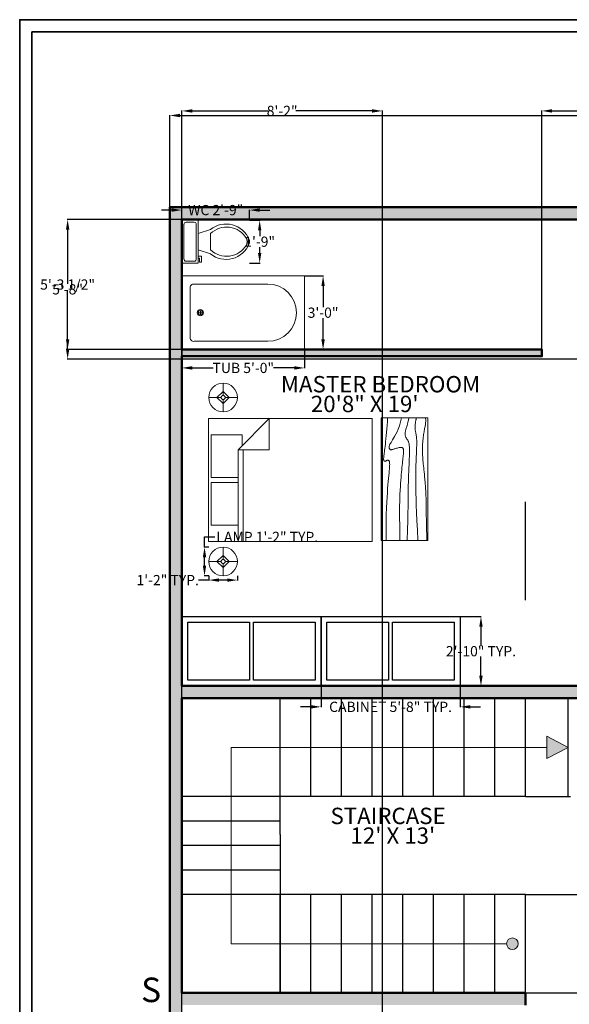
# Model space of a CAD drawing. Units: inches. Extents: x -60 to 743, y -483 to 510.
# Tile 5 of 7: x -60 to 209, y 29 to 510. Entities that reach past the tile are written whole.
import ezdxf

# ---------------------------------------------------------------- set-up
doc = ezdxf.new("R2010")
doc.units = ezdxf.units.IN
doc.header["$MEASUREMENT"] = 0
for name, color, linetype, lineweight in [('A-ANNO-DIMS', 2, 'Continuous', 18), ('A-ANNO-SYMB', 7, 'Continuous', 18), ('A-ANNO-TTLB', 7, 'Continuous', 35), ('A-AREA-IDEN', 7, 'Continuous', 25), ('A-FLOR-CASE', 40, 'Continuous', 25), ('A-FLOR-FIXT', 40, 'Continuous', 18), ('A-WALL-PATT', 30, 'Continuous', 13), ('FURNITURE', 40, 'Continuous', 18), ('STAIRS', 202, 'Continuous', 25), ('WALL BOUNDRY', 10, 'Continuous', 50)]:
    doc.layers.add(name, color=color, linetype=linetype, lineweight=lineweight)
doc.styles.get("Standard").update_dxf_attribs({"font": 'arial.ttf'})
doc.dimstyles.get("Standard").update_dxf_attribs({"dimtxt": 5, "dimasz": 5, "dimexe": 0.18, "dimexo": 0.0625, "dimgap": 0.09, "dimtad": 0, "dimtih": 1, "dimtoh": 1, "dimdec": 1, "dimzin": 0, "dimdsep": 46, "dimlunit": 4, "dimtxsty": 'Standard', "dimcen": 0.09, "dimadec": 0, "dimazin": 0, "dimtfac": 1, "dimtdec": 1, "dimtofl": 0, "dimtmove": 0, "dimatfit": 3, "dimfxl": 1, "dimtolj": 1, "dimtzin": 0, "dimarcsym": 0})

# ---------------------------------------------------------------- blocks, each defined once
blk = doc.blocks.new('Wall Cabinet - 18 x 36 in front')
for p, q in [((17.5, -1.5), (17.5, -16.5)), ((18.5, -16.5), (18.5, -1.5))]:
    blk.add_line(p, q)
blk.add_lwpolyline([(0, -18), (0, 0), (36, 0), (36, -18)], close=True)
for points in [[(17.5, -16.5), (1.5, -16.5), (1.5, -1.5), (17.5, -1.5)], [(18.5, -1.5), (34.5, -1.5), (34.5, -16.5), (18.5, -16.5)]]:
    blk.add_lwpolyline(points)
blk = doc.blocks.new('Bath Tub - 26 x 60 in.')
for p, q in [((8, -18), (10, -18)), ((9, -17), (9, -19))]:
    blk.add_line(p, q)
blk.add_lwpolyline([(0, -36), (0, 0), (60, 0), (60, -36)], close=True)
for points in [[(6, -4), (42, -4)], [(4, -30), (4, -6)], [(42, -32), (6, -32)]]:
    blk.add_lwpolyline(points)
for radius in [1.5, 1]:
    blk.add_circle((9, -18), radius)
for centre, radius, start, end in [((5.75, -5.75), 1.77, 81.8699, 188.1301), ((42, -18), 14, 270, 90), ((5.75, -30.25), 1.77, 171.8699, 278.1301)]:
    blk.add_arc(centre, radius, start, end)
blk = doc.blocks.new('Toilet - top')
for p, q in [((9.5, -6), (9.5, -2)), ((-10, -8.5), (-8, -8.5)), ((-10, -9.5), (-10, -8.5)), ((-7, -9.5), (-10, -9.5)), ((-8, -8.5), (-8, -8)), ((-7, -8), (-7, -9.5)), ((-4, -8), (-6, -14)), ((4, -8), (6, -14)), ((4, -14), (-4, -14))]:
    blk.add_line(p, q)
blk.add_lwpolyline([(10.5, -8), (10.5, 0), (-10.5, 0), (-10.5, -8)], close=True)
for points in [[(-9.5, -2), (-9.5, -6)], [(8.5, -1), (-8.5, -1)], [(-8.5, -7), (8.5, -7)]]:
    blk.add_lwpolyline(points)
for centre, radius, start, end in [((-8.62, -1.88), 0.884, 81.8699, 188.1301), ((8.62, -1.88), 0.884, 351.8699, 98.1301), ((-8.62, -6.12), 0.884, 171.8699, 278.1301), ((8.62, -6.12), 0.884, 261.8699, 8.1301), ((3.52, -21.58), 12.17, 141.4691, 247.9714), ((4.2, -21.82), 11.33, 136.3677, 238.9468), ((-3.52, -21.58), 12.17, 292.0284, 38.5307), ((-4.2, -21.82), 11.33, 301.053, 43.6321), ((0, -27.88), 4, 245.7318, 294.2682), ((0, -29), 4, 254.8605, 285.1395)]:
    blk.add_arc(centre, radius, start, end)
blk = doc.blocks.new('Lamp - Table')
for p, q in [((0, 7), (0, 1)), ((-1, 0), (-7, 0)), ((0, 3), (-3, 0)), ((-3, 0), (0, -3)), ((3, 0), (0, 3)), ((0, -3), (3, 0)), ((1, 0), (7, 0)), ((0, -1), (0, -7))]:
    blk.add_line(p, q)
for radius in [7, 1]:
    blk.add_circle((0, 0), radius)
blk = doc.blocks.new('Bed - Queen')
for p, q in [((0, -80.00003), (0, 0)), ((0, 0), (59.99999, 0)), ((59.99999, 0), (59.99999, -80.00003)), ((7.99999, -1.2), (28.79998, -1.2)), ((7.99999, -14.4), (7.99999, -1.2)), ((28.79998, -1.2), (28.79998, -14.4)), ((31.19999, -1.2), (51.99999, -1.2)), ((31.19999, -14.4), (31.19999, -1.2)), ((51.99999, -1.2), (51.99999, -16.4)), ((0, -14.4), (44.8, -14.4)), ((59.99999, -29.6), (44.8, -14.4)), ((44.8, -14.4), (44.8, -29.6)), ((44.8, -16.8), (0, -16.8)), ((51.99999, -16.4), (46.79936, -16.4)), ((44.8, -29.6), (59.99999, -29.6)), ((59.99999, -80.00003), (0, -80.00003))]:
    blk.add_line(p, q)
blk = doc.blocks.new('*D22')
at = {"layer": 'A-ANNO-DIMS', "color": 0, "lineweight": -2, "transparency": 16777216}
for p, q in [((13.15, 418.48), (13.15, 463.48)), ((18.15, 463.3), (310.31, 463.3)), ((611.15, 463.3), (318.98, 463.3)), ((616.15, 418.48), (616.15, 463.48))]:
    blk.add_line(p, q, dxfattribs=at)
at = {"layer": 'A-ANNO-DIMS', "color": 0, "transparency": 16777216}
for points in [[(18.15, 464.13), (18.15, 462.46), (13.15, 463.3)], [(611.15, 464.13), (611.15, 462.46), (616.15, 463.3)]]:
    blk.add_solid(points, dxfattribs=at)
at = {"layer": 'Defpoints', "color": 0, "transparency": 16777216}
for p in [(616.15, 463.3), (13.15, 418.42), (616.15, 418.42)]:
    blk.add_point(p, dxfattribs=at)
at = {"layer": 'A-ANNO-DIMS', "color": 0, "transparency": 16777216, "insert": (314.65, 463.3), "char_height": 5, "attachment_point": 5}
blk.add_mtext("\\A1;50'", dxfattribs=at)
blk = doc.blocks.new('BENCH-WOOD-60IN')
blk.add_lwpolyline([(22.9143, 0), (22.9143, 60), (0, 60), (0, 0)], close=True)
for points in [[(2.4, 0), (2.418, 4.8155), (2.4688, 9.0302), (2.5477, 12.709), (2.65, 15.9167), (2.7711, 18.7181), (2.9063, 21.1781), (3.0508, 23.3616), (3.2, 25.3333), (3.3495, 27.1477), (3.4958, 28.8172), (3.636, 30.3437), (3.7667, 31.7291), (3.8849, 32.9756), (3.9875, 34.0849), (4.0714, 35.059), (4.1334, 35.9), (4.1711, 36.6114), (4.1854, 37.2041), (4.1779, 37.6906), (4.15, 38.0833), (4.1034, 38.3948), (4.0396, 38.6375), (3.9602, 38.8239), (3.8667, 38.9666), (3.7608, 39.0764), (3.6448, 39.1573), (3.521, 39.2116), (3.3917, 39.2416), (3.2593, 39.2498), (3.1261, 39.2385), (2.9944, 39.21), (2.8667, 39.1666), (2.7447, 39.111), (2.6281, 39.0468), (2.5163, 38.978), (2.4083, 38.9083), (2.3035, 38.8418), (2.201, 38.7823), (2.1001, 38.7337), (2, 38.7), (1.9003, 38.6844), (1.8021, 38.6875), (1.707, 38.7094), (1.6167, 38.75), (1.5326, 38.8094), (1.4563, 38.8875), (1.3893, 38.9844), (1.3333, 39.1), (1.2896, 39.2351), (1.2583, 39.3937), (1.2396, 39.5804), (1.2333, 39.8), (1.2396, 40.057), (1.2583, 40.3562), (1.2896, 40.7023), (1.3333, 41.1), (1.3895, 41.5547), (1.4573, 42.0755), (1.5361, 42.6721), (1.625, 43.3542), (1.7233, 44.1316), (1.8302, 45.014), (1.9449, 46.0114), (2.0667, 47.1333), (2.1947, 48.3862), (2.3281, 49.7625), (2.4663, 51.2513), (2.6083, 52.8416), (2.7535, 54.5226), (2.9011, 56.2833), (3.0501, 58.1127), (3.2, 60)], [(9.2, 0), (9.0858, 6.5759), (9.0365, 11.9385), (9.0418, 16.2527), (9.0917, 19.6833), (9.1759, 22.3952), (9.2844, 24.5531), (9.4069, 26.322), (9.5333, 27.8666), (9.6553, 29.3241), (9.7719, 30.7203), (9.8837, 32.0532), (9.9917, 33.3208), (10.0965, 34.5213), (10.199, 35.6526), (10.2999, 36.7128), (10.4, 37.7), (10.4996, 38.6129), (10.5969, 39.4531), (10.6895, 40.223), (10.775, 40.925), (10.8512, 41.5613), (10.9156, 42.1344), (10.966, 42.6465), (11, 43.1), (11.0158, 43.4976), (11.0136, 43.8437), (10.9942, 44.143), (10.9583, 44.4), (10.9069, 44.6195), (10.8406, 44.8062), (10.7603, 44.9648), (10.6667, 45.1), (10.5598, 45.2155), (10.4365, 45.3114), (10.2929, 45.3871), (10.125, 45.4416), (9.929, 45.4743), (9.7011, 45.4844), (9.4371, 45.4709), (9.1333, 45.4333), (8.7883, 45.3716), (8.4104, 45.2896), (8.0107, 45.1919), (7.6, 45.0833), (7.1893, 44.9685), (6.7896, 44.8521), (6.4117, 44.7388), (6.0667, 44.6333), (5.7628, 44.54), (5.4979, 44.4614), (5.2675, 44.4001), (5.0667, 44.3583), (4.8909, 44.3384), (4.7354, 44.3427), (4.5956, 44.3736), (4.4667, 44.4333), (4.3453, 44.5236), (4.2333, 44.6427), (4.1339, 44.7884), (4.05, 44.9583), (3.9849, 45.1501), (3.9417, 45.3614), (3.9234, 45.59), (3.9333, 45.8333), (3.9749, 46.0915), (4.0531, 46.3734), (4.1736, 46.6906), (4.3417, 47.0542), (4.5629, 47.4756), (4.8427, 47.9661), (5.1866, 48.5372), (5.6, 49.2), (6.0844, 49.9676), (6.625, 50.8594), (7.2031, 51.8965), (7.8, 53.1), (8.3969, 54.491), (8.975, 56.0906), (9.5156, 57.9199), (10, 60)], [(12.8, 0), (12.9322, 5.1847), (13.0323, 9.6213), (13.1059, 13.3963), (13.1583, 16.5958), (13.1952, 19.3063), (13.2219, 21.614), (13.2439, 23.6054), (13.2667, 25.3666), (13.2947, 26.9728), (13.3281, 28.4531), (13.3663, 29.8256), (13.4083, 31.1083), (13.4535, 32.3191), (13.501, 33.476), (13.5501, 34.597), (13.6, 35.7), (13.6497, 36.7984), (13.6979, 37.8875), (13.743, 38.9578), (13.7833, 40), (13.8174, 41.0047), (13.8438, 41.9625), (13.8607, 42.864), (13.8667, 43.7), (13.8604, 44.4631), (13.8417, 45.1552), (13.8104, 45.7801), (13.7667, 46.3416), (13.7104, 46.8439), (13.6417, 47.2906), (13.5604, 47.6858), (13.4667, 48.0333), (13.3608, 48.3375), (13.2448, 48.6042), (13.121, 48.8396), (12.9917, 49.05), (12.8593, 49.2417), (12.7261, 49.4208), (12.5944, 49.5937), (12.4667, 49.7667), (12.3451, 49.9452), (12.2313, 50.1323), (12.1268, 50.3303), (12.0333, 50.5416), (11.9524, 50.7686), (11.8854, 51.0135), (11.8341, 51.2788), (11.8, 51.5666), (11.7843, 51.8785), (11.7865, 52.2116), (11.8059, 52.562), (11.8417, 52.926), (11.8931, 53.2998), (11.9594, 53.6795), (12.0397, 54.0614), (12.1333, 54.4416), (12.2401, 54.8223), (12.3625, 55.2293), (12.5037, 55.6942), (12.6667, 56.2489), (12.8547, 56.9251), (13.0708, 57.7545), (13.3182, 58.7689), (13.6, 60)], [(18, 0), (17.7273, 5.124), (17.5057, 9.6609), (17.3303, 13.6705), (17.1958, 17.2125), (17.0973, 20.3467), (17.0297, 23.1328), (16.9878, 25.6307), (16.9667, 27.9), (16.9617, 29.9928), (16.9703, 31.9302), (16.9907, 33.7254), (17.0208, 35.3917), (17.0588, 36.9423), (17.1026, 38.3906), (17.1503, 39.7499), (17.2, 41.0333), (17.2496, 42.2519), (17.2969, 43.4073), (17.3395, 44.4986), (17.375, 45.525), (17.4012, 46.4858), (17.4156, 47.3802), (17.416, 48.2074), (17.4, 48.9667), (17.3662, 49.6583), (17.3167, 50.2872), (17.2547, 50.8595), (17.1833, 51.3812), (17.1057, 51.8584), (17.025, 52.2971), (16.9443, 52.7034), (16.8667, 53.0833), (16.7951, 53.443), (16.7313, 53.789), (16.6768, 54.128), (16.6334, 54.4666), (16.6024, 54.8115), (16.5854, 55.1693), (16.5841, 55.5465), (16.6, 55.95), (16.6337, 56.3828), (16.6823, 56.8346), (16.7418, 57.2915), (16.8084, 57.7396), (16.878, 58.165), (16.9469, 58.5539), (17.0111, 58.8924), (17.0667, 59.1666), (17.1107, 59.3679), (17.1438, 59.5078), (17.1675, 59.6032), (17.1833, 59.6708), (17.193, 59.7275), (17.1979, 59.7901), (17.1998, 59.8753), (17.2, 60)], [(22.4, 0), (22.2501, 8.0098), (22.1011, 14.4094), (21.9535, 19.4168), (21.8083, 23.25), (21.6663, 26.1269), (21.5281, 28.2656), (21.3947, 29.884), (21.2667, 31.2), (21.1448, 32.3967), (21.0292, 33.5172), (20.9198, 34.5697), (20.8167, 35.5625), (20.7198, 36.5037), (20.6292, 37.4015), (20.5448, 38.2642), (20.4667, 39.1), (20.3951, 39.9164), (20.3313, 40.7187), (20.2768, 41.5117), (20.2333, 42.3), (20.2024, 43.0883), (20.1854, 43.8812), (20.1841, 44.6836), (20.2, 45.5), (20.234, 46.3328), (20.2844, 47.1747), (20.3488, 48.0163), (20.425, 48.8479), (20.5106, 49.66), (20.6031, 50.4429), (20.7004, 51.1872), (20.8, 51.8833), (20.8999, 52.5246), (20.9995, 53.1166), (21.0983, 53.6681), (21.1958, 54.1875), (21.2919, 54.6834), (21.3859, 55.1646), (21.4777, 55.6394), (21.5667, 56.1167), (21.6515, 56.6028), (21.7266, 57.0961), (21.7852, 57.5929), (21.8208, 58.0896), (21.8268, 58.5823), (21.7964, 59.0674), (21.723, 59.5412), (21.6, 60)]]:
    blk.add_lwpolyline(points)
blk = doc.blocks.new('*D28')
at = {"layer": 'A-ANNO-DIMS', "color": 0, "lineweight": -2, "transparency": 16777216}
for p, q in [((87.15, 184.36), (87.15, 174.04)), ((155.15, 184.36), (155.15, 174.04)), ((82.15, 174.22), (77.15, 174.22)), ((160.15, 174.22), (165.15, 174.22))]:
    blk.add_line(p, q, dxfattribs=at)
at = {"layer": 'A-ANNO-DIMS', "color": 0, "transparency": 16777216}
for points in [[(82.15, 175.05), (82.15, 173.39), (87.15, 174.22)], [(160.15, 175.05), (160.15, 173.39), (155.15, 174.22)]]:
    blk.add_solid(points, dxfattribs=at)
at = {"layer": 'Defpoints', "color": 0, "transparency": 16777216}
for p in [(87.15, 184.42), (155.15, 184.42), (155.15, 174.22)]:
    blk.add_point(p, dxfattribs=at)
at = {"layer": 'A-ANNO-DIMS', "color": 0, "transparency": 16777216, "insert": (121.15, 174.22), "char_height": 5, "attachment_point": 5}
blk.add_mtext('\\A1;CABINET 5\'-8" TYP.', dxfattribs=at)
blk = doc.blocks.new('*D29')
at = {"layer": 'A-ANNO-DIMS', "color": 0, "lineweight": -2, "transparency": 16777216}
for p, q in [((155.22, 218.42), (165.53, 218.42)), ((165.35, 213.42), (165.35, 204.07)), ((165.35, 189.42), (165.35, 198.78)), ((155.22, 184.42), (165.53, 184.42))]:
    blk.add_line(p, q, dxfattribs=at)
at = {"layer": 'A-ANNO-DIMS', "color": 0, "transparency": 16777216}
for points in [[(164.52, 213.42), (166.19, 213.42), (165.35, 218.42)], [(164.52, 189.42), (166.19, 189.42), (165.35, 184.42)]]:
    blk.add_solid(points, dxfattribs=at)
at = {"layer": 'Defpoints', "color": 0, "transparency": 16777216}
for p in [(155.15, 218.42), (165.35, 218.42), (155.15, 184.42)]:
    blk.add_point(p, dxfattribs=at)
at = {"layer": 'A-ANNO-DIMS', "color": 0, "transparency": 16777216, "insert": (165.35, 201.42), "char_height": 5, "attachment_point": 5}
blk.add_mtext('\\A1;2\'-10" TYP.', dxfattribs=at)
blk = doc.blocks.new('*D32')
at = {"layer": 'A-ANNO-DIMS', "color": 0, "lineweight": -2, "transparency": 16777216}
for p, q in [((30.18, 252.28), (30.18, 257.28)), ((30.18, 257.28), (35.18, 257.28)), ((32.22, 252.28), (30, 252.28)), ((30.18, 243.28), (30.18, 247.28)), ((32.22, 238.28), (30, 238.28))]:
    blk.add_line(p, q, dxfattribs=at)
at = {"layer": 'A-ANNO-DIMS', "color": 0, "transparency": 16777216}
for points in [[(29.35, 247.28), (31.01, 247.28), (30.18, 252.28)], [(29.35, 243.28), (31.01, 243.28), (30.18, 238.28)]]:
    blk.add_solid(points, dxfattribs=at)
at = {"layer": 'Defpoints', "color": 0, "transparency": 16777216}
for p in [(30.18, 252.28), (32.28, 252.28), (32.28, 238.28)]:
    blk.add_point(p, dxfattribs=at)
at = {"layer": 'A-ANNO-DIMS', "color": 0, "transparency": 16777216, "insert": (60.88, 257.28), "char_height": 5, "attachment_point": 5}
blk.add_mtext('\\A1;LAMP 1\'-2" TYP.', dxfattribs=at)
blk = doc.blocks.new('*D33')
at = {"layer": 'A-ANNO-DIMS', "color": 0, "lineweight": -2, "transparency": 16777216}
for p, q in [((32.28, 236.18), (27.28, 236.18)), ((32.28, 238.22), (32.28, 236)), ((41.28, 236.18), (37.28, 236.18)), ((46.28, 238.22), (46.28, 236))]:
    blk.add_line(p, q, dxfattribs=at)
at = {"layer": 'A-ANNO-DIMS', "color": 0, "transparency": 16777216}
for points in [[(37.28, 237.01), (37.28, 235.35), (32.28, 236.18)], [(41.28, 237.01), (41.28, 235.35), (46.28, 236.18)]]:
    blk.add_solid(points, dxfattribs=at)
at = {"layer": 'Defpoints', "color": 0, "transparency": 16777216}
for p in [(32.28, 238.28), (32.28, 236.18), (46.28, 238.28)]:
    blk.add_point(p, dxfattribs=at)
at = {"layer": 'A-ANNO-DIMS', "color": 0, "transparency": 16777216, "insert": (12.19, 236.18), "char_height": 5, "attachment_point": 5}
blk.add_mtext('\\A1;1\'-2" TYP.', dxfattribs=at)
blk = doc.blocks.new('*D38')
at = {"layer": 'A-ANNO-DIMS', "color": 0, "lineweight": -2, "transparency": 16777216}
for p, q in [((19.15, 348.84), (19.15, 339.72)), ((79.15, 348.84), (79.15, 339.72)), ((24.15, 339.9), (34.39, 339.9)), ((74.15, 339.9), (63.9, 339.9))]:
    blk.add_line(p, q, dxfattribs=at)
at = {"layer": 'A-ANNO-DIMS', "color": 0, "transparency": 16777216}
for points in [[(24.15, 340.73), (24.15, 339.07), (19.15, 339.9)], [(74.15, 340.73), (74.15, 339.07), (79.15, 339.9)]]:
    blk.add_solid(points, dxfattribs=at)
at = {"layer": 'Defpoints', "color": 0, "transparency": 16777216}
for p in [(19.15, 348.9), (79.15, 348.9), (79.15, 339.9)]:
    blk.add_point(p, dxfattribs=at)
at = {"layer": 'A-ANNO-DIMS', "color": 0, "transparency": 16777216, "insert": (49.15, 339.9), "char_height": 5, "attachment_point": 5}
blk.add_mtext('\\A1;TUB 5\'-0"', dxfattribs=at)
blk = doc.blocks.new('*D39')
at = {"layer": 'A-ANNO-DIMS', "color": 0, "lineweight": -2, "transparency": 16777216}
for p, q in [((79.21, 384.9), (88.33, 384.9)), ((88.15, 379.9), (88.15, 369.54)), ((88.15, 353.9), (88.15, 364.26)), ((79.21, 348.9), (88.33, 348.9))]:
    blk.add_line(p, q, dxfattribs=at)
at = {"layer": 'A-ANNO-DIMS', "color": 0, "transparency": 16777216}
for points in [[(87.31, 379.9), (88.98, 379.9), (88.15, 384.9)], [(87.31, 353.9), (88.98, 353.9), (88.15, 348.9)]]:
    blk.add_solid(points, dxfattribs=at)
at = {"layer": 'Defpoints', "color": 0, "transparency": 16777216}
for p in [(79.15, 384.9), (88.15, 384.9), (79.15, 348.9)]:
    blk.add_point(p, dxfattribs=at)
at = {"layer": 'A-ANNO-DIMS', "color": 0, "transparency": 16777216, "insert": (88.15, 366.9), "char_height": 5, "attachment_point": 5}
blk.add_mtext('\\A1;3\'-0"', dxfattribs=at)
blk = doc.blocks.new('*D44')
at = {"layer": 'A-ANNO-DIMS', "color": 0, "lineweight": -2, "transparency": 16777216}
for p, q in [((14.15, 417.05), (9.15, 417.05)), ((19.15, 412.16), (19.15, 417.23)), ((52.19, 412.16), (52.19, 417.23)), ((57.19, 417.05), (62.19, 417.05))]:
    blk.add_line(p, q, dxfattribs=at)
at = {"layer": 'A-ANNO-DIMS', "color": 0, "transparency": 16777216}
for points in [[(14.15, 417.89), (14.15, 416.22), (19.15, 417.05)], [(57.19, 417.89), (57.19, 416.22), (52.19, 417.05)]]:
    blk.add_solid(points, dxfattribs=at)
at = {"layer": 'Defpoints', "color": 0, "transparency": 16777216}
for p in [(19.15, 417.05), (19.15, 412.1), (52.19, 412.1)]:
    blk.add_point(p, dxfattribs=at)
at = {"layer": 'A-ANNO-DIMS', "color": 0, "transparency": 16777216, "insert": (35.67, 417.05), "char_height": 5, "attachment_point": 5}
blk.add_mtext('\\A1;WC 2\'-9"', dxfattribs=at)
blk = doc.blocks.new('*D45')
at = {"layer": 'A-ANNO-DIMS', "color": 0, "lineweight": -2, "transparency": 16777216}
for p, q in [((52.26, 412.1), (57.33, 412.1)), ((57.15, 407.1), (57.15, 404.24)), ((57.15, 396.1), (57.15, 398.95)), ((52.26, 391.1), (57.33, 391.1))]:
    blk.add_line(p, q, dxfattribs=at)
at = {"layer": 'A-ANNO-DIMS', "color": 0, "transparency": 16777216}
for points in [[(56.32, 407.1), (57.98, 407.1), (57.15, 412.1)], [(56.32, 396.1), (57.98, 396.1), (57.15, 391.1)]]:
    blk.add_solid(points, dxfattribs=at)
at = {"layer": 'Defpoints', "color": 0, "transparency": 16777216}
for p in [(52.19, 412.1), (57.15, 412.1), (52.19, 391.1)]:
    blk.add_point(p, dxfattribs=at)
at = {"layer": 'A-ANNO-DIMS', "color": 0, "transparency": 16777216, "insert": (57.15, 401.6), "char_height": 5, "attachment_point": 5}
blk.add_mtext('\\A1;1\'-9"', dxfattribs=at)
blk = doc.blocks.new('*D68')
at = {"layer": 'A-ANNO-DIMS', "color": 0, "lineweight": -2, "transparency": 16777216}
for p, q in [((273.08, 412.42), (-36.93, 412.42)), ((-36.75, 407.42), (-36.75, 380.97)), ((-36.75, 349.23), (-36.75, 375.68)), ((273.08, 344.23), (-36.93, 344.23))]:
    blk.add_line(p, q, dxfattribs=at)
at = {"layer": 'A-ANNO-DIMS', "color": 0, "transparency": 16777216}
for points in [[(-37.58, 407.42), (-35.91, 407.42), (-36.75, 412.42)], [(-37.58, 349.23), (-35.91, 349.23), (-36.75, 344.23)]]:
    blk.add_solid(points, dxfattribs=at)
at = {"layer": 'Defpoints', "color": 0, "transparency": 16777216}
for p in [(273.15, 412.42), (-36.75, 344.23), (273.15, 344.23)]:
    blk.add_point(p, dxfattribs=at)
at = {"layer": 'A-ANNO-DIMS', "color": 0, "transparency": 16777216, "insert": (-36.75, 378.32), "char_height": 5, "attachment_point": 5}
blk.add_mtext('\\A1;5\'-8"', dxfattribs=at)
blk = doc.blocks.new('*D73')
at = {"layer": 'A-ANNO-DIMS', "color": 0, "lineweight": -2, "transparency": 16777216}
for p, q in [((19.15, -143.52), (19.15, 465.7)), ((24.15, 465.52), (61.41, 465.52)), ((112.15, 465.52), (74.89, 465.52)), ((117.15, -143.52), (117.15, 465.7))]:
    blk.add_line(p, q, dxfattribs=at)
at = {"layer": 'A-ANNO-DIMS', "color": 0, "transparency": 16777216}
for points in [[(24.15, 466.36), (24.15, 464.69), (19.15, 465.52)], [(112.15, 466.36), (112.15, 464.69), (117.15, 465.52)]]:
    blk.add_solid(points, dxfattribs=at)
at = {"layer": 'Defpoints', "color": 0, "transparency": 16777216}
for p in [(117.15, 465.52), (19.15, -143.58), (117.15, -143.58)]:
    blk.add_point(p, dxfattribs=at)
at = {"layer": 'A-ANNO-DIMS', "color": 0, "transparency": 16777216, "insert": (68.15, 465.52), "char_height": 5, "attachment_point": 5}
blk.add_mtext('\\A1;8\'-2"', dxfattribs=at)
blk = doc.blocks.new('*D74')
at = {"layer": 'A-ANNO-DIMS', "color": 0, "lineweight": -2, "transparency": 16777216}
for p, q in [((187.21, 82.42), (679.73, 82.42)), ((679.55, 77.42), (679.55, 61.06)), ((679.55, 39.42), (679.55, 55.78)), ((187.21, 34.42), (679.73, 34.42))]:
    blk.add_line(p, q, dxfattribs=at)
at = {"layer": 'A-ANNO-DIMS', "color": 0, "transparency": 16777216}
for points in [[(678.72, 77.42), (680.39, 77.42), (679.55, 82.42)], [(678.72, 39.42), (680.39, 39.42), (679.55, 34.42)]]:
    blk.add_solid(points, dxfattribs=at)
at = {"layer": 'Defpoints', "color": 0, "transparency": 16777216}
for p in [(187.15, 82.42), (679.55, 82.42), (187.15, 34.42)]:
    blk.add_point(p, dxfattribs=at)
at = {"layer": 'A-ANNO-DIMS', "color": 0, "transparency": 16777216, "insert": (679.55, 58.42), "char_height": 5, "attachment_point": 5}
blk.add_mtext('\\A1;4\'-0"', dxfattribs=at)
blk = doc.blocks.new('*D80')
at = {"layer": 'A-ANNO-DIMS', "color": 0, "lineweight": -2, "transparency": 16777216}
for p, q in [((19.08, 412.42), (-36.93, 412.42)), ((-36.75, 407.42), (-36.75, 383.34)), ((-36.75, 353.9), (-36.75, 377.98)), ((19.08, 348.9), (-36.93, 348.9))]:
    blk.add_line(p, q, dxfattribs=at)
at = {"layer": 'A-ANNO-DIMS', "color": 0, "transparency": 16777216}
for points in [[(-37.58, 407.42), (-35.91, 407.42), (-36.75, 412.42)], [(-37.58, 353.9), (-35.91, 353.9), (-36.75, 348.9)]]:
    blk.add_solid(points, dxfattribs=at)
at = {"layer": 'Defpoints', "color": 0, "transparency": 16777216}
for p in [(19.15, 412.42), (-36.75, 348.9), (19.15, 348.9)]:
    blk.add_point(p, dxfattribs=at)
at = {"layer": 'A-ANNO-DIMS', "color": 0, "transparency": 16777216, "insert": (-36.75, 380.66), "char_height": 5, "attachment_point": 5}
blk.add_mtext('\\A1;5\'-3 1/2"', dxfattribs=at)
blk = doc.blocks.new('*D81')
at = {"layer": 'A-ANNO-DIMS', "color": 0, "lineweight": -2, "transparency": 16777216}
for p, q in [((195.14, 348.96), (195.14, 465.7)), ((200.14, 465.52), (224.39, 465.52)), ((262.15, 465.52), (237.89, 465.52)), ((267.15, 412.48), (267.15, 465.7))]:
    blk.add_line(p, q, dxfattribs=at)
at = {"layer": 'A-ANNO-DIMS', "color": 0, "transparency": 16777216}
for points in [[(200.14, 466.36), (200.14, 464.69), (195.14, 465.52)], [(262.15, 466.36), (262.15, 464.69), (267.15, 465.52)]]:
    blk.add_solid(points, dxfattribs=at)
at = {"layer": 'Defpoints', "color": 0, "transparency": 16777216}
for p in [(267.15, 465.52), (267.15, 412.42), (195.14, 348.9)]:
    blk.add_point(p, dxfattribs=at)
at = {"layer": 'A-ANNO-DIMS', "color": 0, "transparency": 16777216, "insert": (231.14, 465.52), "char_height": 5, "attachment_point": 5}
blk.add_mtext('\\A1;6\'-0"', dxfattribs=at)

msp = doc.modelspace()

# ---------------------------------------------------------------- hatches: boundary and pattern name
at = {"layer": 'A-ANNO-SYMB'}
h = msp.add_hatch(color=256, dxfattribs=at)
h.dxf.hatch_style = 1
h.paths.add_polyline_path([(207.98, 154.42), (197.62, 159.82), (197.62, 154.42), (197.62, 149.03)])
h.paths.add_polyline_path([(183.55, 58.42, 1), (177.89, 58.42, 1)])
at = {"layer": 'A-WALL-PATT'}
h = msp.add_hatch(color=256, dxfattribs=at)
h.dxf.hatch_style = 1
h.paths.add_polyline_path([(412.35, 168.77), (415.89, 168.77), (415.89, 114.92), (412.35, 114.92)], flags=16)
h.paths.add_polyline_path([(87.81, -138.81), (87.81, -142.35), (48.31, -142.32), (48.31, -138.78)], flags=16)
h.paths.add_polyline_path([(459.53, -138.78), (513.39, -138.78), (513.39, -142.32), (459.53, -142.32)], flags=16)
h.paths.add_polyline_path([(164.84, -257.78), (218.7, -257.78), (218.7, -261.32), (164.84, -261.32)], flags=16)
h.paths.add_polyline_path([(417.15, 114.92), (415.89, 114.92), (415.89, 168.77), (417.15, 168.77), (417.15, 195.42), (411.15, 195.42), (411.15, 168.77), (412.35, 168.77), (412.35, 114.92), (411.15, 114.92), (411.15, 28.42), (610.15, 28.42), (610.15, -43.58), (508.15, -43.58), (508.15, -49.58), (610.15, -49.58), (610.15, -137.58), (513.39, -137.58), (513.39, -138.78), (459.53, -138.78), (459.53, -137.58), (359.15, -137.58), (359.15, -143.58), (377.15, -143.58), (377.15, -292.58), (383.15, -292.58), (383.15, -143.58), (459.53, -143.58), (459.53, -142.32), (513.39, -142.32), (513.39, -143.58), (610.15, -143.58), (610.15, -415.58), (610.15, -421.58), (616.15, -421.58), (616.15, 418.42), (13.15, 418.42), (13.15, -421.58), (19.15, -421.58), (430.15, -421.58), (430.15, -415.58), (19.15, -415.58), (19.15, -143.58), (48.31, -143.58), (48.31, -142.32), (87.81, -142.35), (87.81, -143.58), (117.15, -143.58), (117.15, -262.58), (164.84, -262.58), (164.84, -261.32), (218.7, -261.32), (218.7, -262.58), (273.15, -262.58), (273.15, -292.58), (279.15, -292.58), (279.15, -143.58), (297.15, -143.58), (297.15, -137.58), (273.15, -137.58), (273.15, -256.58), (218.7, -256.58), (218.7, -257.78), (164.84, -257.78), (164.84, -256.58), (123.15, -256.58), (123.15, -143.58), (225.15, -143.58), (225.15, -137.58), (87.81, -137.58), (87.81, -138.81), (48.31, -138.78), (48.31, -137.58), (19.15, -137.58), (19.15, 28.42), (187.15, 28.42), (187.15, 34.42), (19.15, 34.42), (19.15, 178.42), (273.15, 178.42), (273.15, 184.42), (19.15, 184.42), (19.15, 345.58), (195.14, 345.58), (195.14, 348.9), (19.15, 348.9), (19.15, 412.42), (267.15, 412.42), (267.15, 319.83), (273.15, 319.83), (273.15, 412.42), (411.15, 412.42), (411.15, 376.24), (417.15, 376.24), (417.15, 412.42), (610.15, 412.42), (610.15, 249.42), (411.15, 249.42), (411.15, 243.42), (610.15, 243.42), (610.15, 34.42), (417.15, 34.42)])

# ---------------------------------------------------------------- linework, layer by layer
at = {"layer": 'A-ANNO-SYMB'}
for p, q in [((197.62, 154.42), (197.62, 159.82)), ((197.62, 159.82), (207.98, 154.42)), ((197.62, 154.42), (43.15, 154.42)), ((43.15, 154.42), (43.15, 58.42)), ((197.62, 154.42), (197.62, 149.03)), ((197.62, 149.03), (207.98, 154.42)), ((43.15, 58.42), (177.89, 58.42))]:
    msp.add_line(p, q, dxfattribs=at)
msp.add_circle((180.72, 58.42), 2.83, dxfattribs=at)
at = {"layer": 'A-ANNO-TTLB'}
for points in [[(742.84, -483.31), (-60.19, -483.31), (-60.19, 510.12), (742.84, 510.12)], [(736.84, -477.31), (-54.19, -477.31), (-54.19, 504.12), (736.84, 504.12)]]:
    msp.add_lwpolyline(points, close=True, dxfattribs=at)
at = {"layer": 'STAIRS'}
for p, q in [((187.15, 226.42), (187.15, 274.42)), ((67.15, 111.75), (67.15, 178.42)), ((67.15, 130.42), (67.15, 178.42)), ((82.15, 130.42), (82.15, 178.42)), ((97.15, 130.42), (97.15, 178.42)), ((112.15, 130.42), (112.15, 178.42)), ((127.15, 130.42), (127.15, 178.42)), ((142.15, 130.42), (142.15, 178.42)), ((157.15, 130.42), (157.15, 178.42)), ((172.15, 130.42), (172.15, 178.42)), ((187.15, 130.42), (187.15, 178.42)), ((187.15, 130.42), (187.15, 178.42)), ((207.98, 130.42), (207.98, 178.42)), ((67.15, 130.42), (19.15, 130.42)), ((67.15, 130.42), (19.15, 130.42)), ((187.15, 130.42), (67.15, 130.42)), ((187.15, 130.42), (209.13, 130.42)), ((67.15, 118.42), (19.15, 118.42)), ((67.15, 111.75), (67.15, 34.42)), ((67.15, 106.42), (19.15, 106.42)), ((67.15, 94.42), (19.15, 94.42)), ((187.15, 82.42), (19.15, 82.42)), ((67.15, 82.42), (19.15, 82.42)), ((67.15, 34.42), (67.15, 82.42)), ((82.15, 34.42), (82.15, 82.42)), ((97.15, 34.42), (97.15, 82.42)), ((112.15, 34.42), (112.15, 82.42)), ((127.15, 34.42), (127.15, 82.42)), ((142.15, 34.42), (142.15, 82.42)), ((157.15, 34.42), (157.15, 82.42)), ((172.15, 34.42), (172.15, 82.42)), ((187.15, 34.42), (187.15, 82.42))]:
    msp.add_line(p, q, dxfattribs=at)
at = {"layer": 'WALL BOUNDRY'}
msp.add_lwpolyline([(610.15, -415.58), (610.15, -421.58), (616.15, -421.58), (616.15, 418.42), (13.15, 418.42), (13.15, -421.58), (19.15, -421.58), (430.15, -421.58), (430.15, -415.58), (19.15, -415.58), (19.15, -143.58), (117.15, -143.58), (117.15, -262.58), (273.15, -262.58), (273.15, -292.58), (279.15, -292.58), (377.15, -292.58), (383.15, -292.58), (383.15, -143.58), (610.15, -143.58)], close=True, dxfattribs=at)
msp.add_lwpolyline([(187.15, 28.42), (187.15, 34.42), (19.15, 34.42), (19.15, 178.42), (273.15, 178.42), (273.15, 184.42), (19.15, 184.42), (19.15, 345.58), (195.14, 345.58), (195.14, 348.9), (19.15, 348.9), (19.15, 412.42), (267.15, 412.42), (267.15, 232.42), (273.15, 232.42), (273.15, 412.42), (411.15, 412.42), (411.15, 297.42), (417.15, 297.42), (417.15, 412.42), (610.15, 412.42)], dxfattribs=at)

# ---------------------------------------------------------------- block references
at = {"layer": 'A-FLOR-CASE', "xscale": 1.888986204117192, "yscale": 1.888986204117192, "zscale": 1.888986204117192}
for p in [(19.15, 218.42), (87.15, 218.42)]:
    msp.add_blockref('Wall Cabinet - 18 x 36 in front', p, dxfattribs=at)
at = {"layer": 'A-FLOR-FIXT', "rotation": 90}
msp.add_blockref('Toilet - top', (19.15, 401.6), dxfattribs=at)
at = {"layer": 'A-FLOR-FIXT'}
msp.add_blockref('Bath Tub - 26 x 60 in.', (19.15, 384.9), dxfattribs=at)
at = {"layer": 'FURNITURE', "rotation": 90}
for name, p in [('Lamp - Table', (39.28, 325.43)), ('Bed - Queen', (32.21, 255.11)), ('Lamp - Table', (39.28, 245.28))]:
    msp.add_blockref(name, p, dxfattribs=at)
at = {"layer": 'FURNITURE'}
msp.add_blockref('BENCH-WOOD-60IN', (116.53, 255.55), dxfattribs=at)

# ---------------------------------------------------------------- texts
at = {"layer": 'A-ANNO-SYMB'}
msp.add_text('S ', height=12, dxfattribs=at).set_placement((-0.82, 29.89))
at = {"layer": 'A-AREA-IDEN'}
for s, p in [('MASTER BEDROOM', (67.51, 327.93)), ('      20\'8" X 19\'', (67.51, 318.29)), ('STAIRCASE ', (91.78, 116.91)), ("    12' X 13'", (91.78, 107.27))]:
    msp.add_text(s, height=8, dxfattribs=at).set_placement(p)

# ---------------------------------------------------------------- dimensions: what is measured, and where the dimension line sits
at = {"layer": 'A-ANNO-DIMS'}
for base, p1, p2, picture, middle in [((117.15, 465.52), (19.15, -143.58), (117.15, -143.58), '*D73', (68.15, 465.52)), ((267.15, 465.52), (195.14, 348.9), (267.15, 412.42), '*D81', (231.14, 465.52))]:
    dim = msp.add_linear_dim(base=base, p1=p1, p2=p2, dimstyle='Standard', override={"dimdec": 1, "dimlfac": 1, "dimrnd": 0, "dimzin": 1, "dimdsep": 46, "dimlunit": 4, "dimfrac": 2}, dxfattribs=at)
    dim.commit()
    dim.dimension.update_dxf_attribs({"geometry": picture, "text_midpoint": middle})
for base, p1, p2, text, override, picture, middle in [((616.15, 463.3), (13.15, 418.42), (616.15, 418.42), "50'", {"dimclrd": 0, "dimclre": 0, "dimclrt": 0}, '*D22', (314.65, 463.3)), ((79.15, 339.9), (19.15, 348.9), (79.15, 348.9), 'TUB <>', {"dimdec": 1, "dimlfac": 1, "dimrnd": 0, "dimzin": 1, "dimdsep": 46, "dimlunit": 4, "dimfrac": 2}, '*D38', (49.15, 339.9)), ((155.15, 174.22), (87.15, 184.42), (155.15, 184.42), 'CABINET <> TYP.', {"dimdec": 1, "dimlfac": 1, "dimrnd": 0, "dimzin": 1, "dimdsep": 46, "dimlunit": 4, "dimfrac": 2}, '*D28', (121.15, 174.22))]:
    dim = msp.add_linear_dim(base=base, p1=p1, p2=p2, text=text, dimstyle='Standard', override=override, dxfattribs=at)
    dim.commit()
    dim.dimension.update_dxf_attribs({"geometry": picture, "text_midpoint": middle})
for base, p1, p2, angle, text, picture, middle in [((19.15, 417.05), (52.19, 412.1), (19.15, 412.1), 180, 'WC <>', '*D44', (35.67, 417.05)), ((30.18, 252.28), (32.28, 238.28), (32.28, 252.28), 90, 'LAMP <> TYP.', '*D32', (60.88, 257.28)), ((32.28, 236.18), (46.28, 238.28), (32.28, 238.28), 180, '<> TYP.', '*D33', (12.19, 236.18)), ((165.35, 218.42), (155.15, 184.42), (155.15, 218.42), 90, '<> TYP.', '*D29', (165.35, 201.42))]:
    dim = msp.add_linear_dim(base=base, p1=p1, p2=p2, angle=angle, text=text, dimstyle='Standard', override={"dimdec": 1, "dimlfac": 1, "dimrnd": 0, "dimzin": 1, "dimdsep": 46, "dimlunit": 4, "dimfrac": 2}, dxfattribs=at)
    dim.commit()
    dim.dimension.update_dxf_attribs({"geometry": picture, "text_midpoint": middle})
for base, p1, p2, picture, middle in [((-36.75, 348.9), (19.15, 412.42), (19.15, 348.9), '*D80', (-36.75, 380.66)), ((-36.75, 344.23), (273.15, 412.42), (273.15, 344.23), '*D68', (-36.75, 378.32)), ((57.15, 412.1), (52.19, 391.1), (52.19, 412.1), '*D45', (57.15, 401.6)), ((88.15, 384.9), (79.15, 348.9), (79.15, 384.9), '*D39', (88.15, 366.9)), ((679.55, 82.42), (187.15, 34.42), (187.15, 82.42), '*D74', (679.55, 58.42))]:
    dim = msp.add_linear_dim(base=base, p1=p1, p2=p2, angle=90, dimstyle='Standard', override={"dimdec": 1, "dimlfac": 1, "dimrnd": 0, "dimzin": 1, "dimdsep": 46, "dimlunit": 4, "dimfrac": 2}, dxfattribs=at)
    dim.commit()
    dim.dimension.update_dxf_attribs({"geometry": picture, "text_midpoint": middle})

doc.saveas('drawing.dxf')
